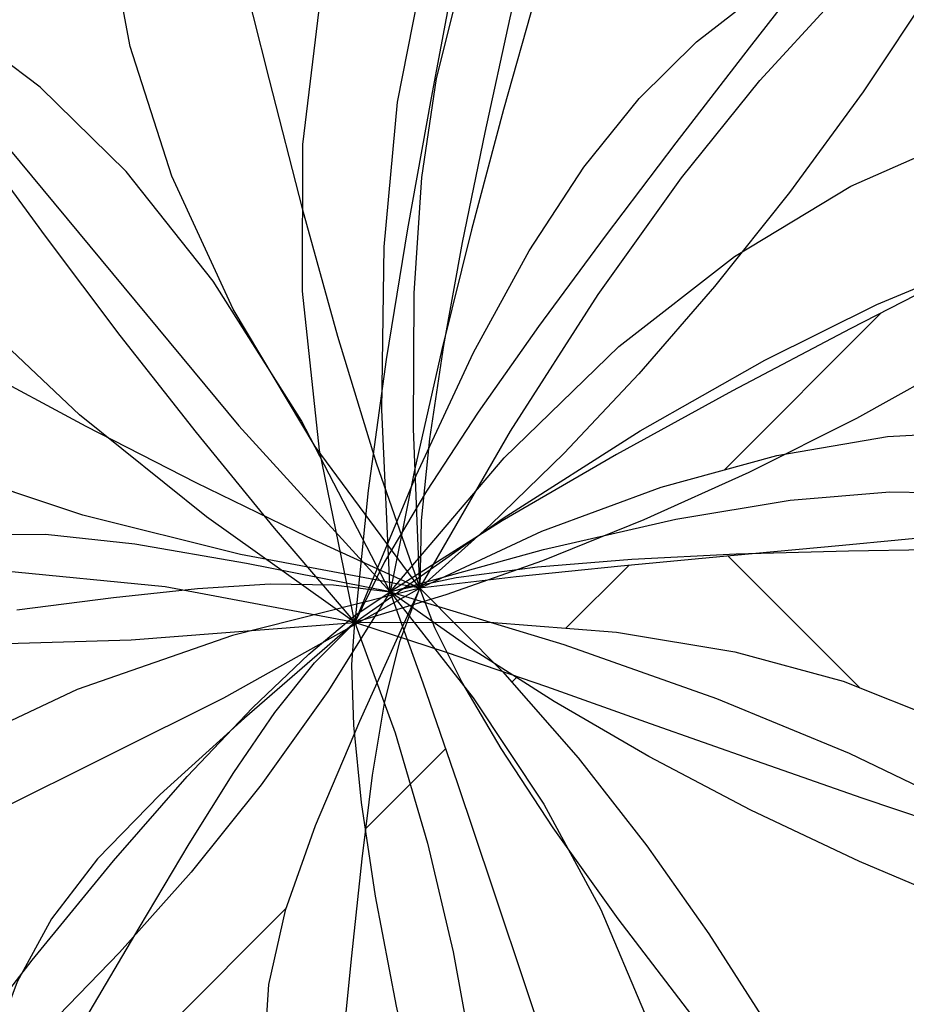
# Model space of a CAD drawing. Units: inches. Extents: x 3590 to 5167, y 65 to 1917.
# Tile 51 of 100: x 4947.17 to 4960.64, y 1515.58 to 1530.53. Entities that reach past the tile are written whole.
import ezdxf

# ---------------------------------------------------------------- set-up
doc = ezdxf.new("R2010")
doc.units = ezdxf.units.IN
doc.layers.add('A-FLOR-PATT', color=8, linetype='Continuous', lineweight=13)
doc.layers.add('L-PLNT', color=94, linetype='Continuous', lineweight=18)
doc.layers.add('DIENHOA', color=3, linetype='Continuous')

# ---------------------------------------------------------------- blocks, each defined once
blk = doc.blocks.new('Cay03_mb')
at = {"layer": 'DIENHOA'}
for p, q in [((9.94, 295.25), (25.49, 374.33)), ((96.72, 365.58), (75.6, 290.61)), ((-211.19, 304.6), (-263.5, 343.48)), ((-158.04, 252.34), (-211.19, 304.6)), ((1.62, 205.66), (9.94, 295.25)), ((75.6, 290.61), (55.75, 216.28)), ((-240.22, 277.83), (-88.39, 94.86)), ((290.63, 243.24), (363.38, 275.41)), ((-104.15, 184.39), (-158.04, 252.34)), ((218.51, 199.79), (290.63, 243.24)), ((55.75, 216.28), (37.33, 142.09)), ((0.21, 104.88), (1.62, 205.66)), ((146.96, 144.09), (218.51, 199.79)), ((363.69, 192.89), (290.19, 154.87)), ((-49.64, 98.45), (-104.15, 184.39)), ((290.19, 154.87), (217.38, 116.61)), ((37.33, 142.09), (20.49, 67.57)), ((75.94, 75.22), (146.96, 144.09)), ((217.38, 116.61), (145.48, 77.28)), ((5.39, -7.78), (0.21, 104.88)), ((5.39, -7.78), (-49.64, 98.45)), ((-88.39, 94.86), (5.39, -7.78)), ((5.39, -7.78), (75.94, 75.22)), ((145.48, 77.28), (74.74, 36.09)), ((20.49, 67.57), (5.39, -7.78)), ((182.2, 37.2), (252.97, 48.94)), ((252.97, 48.94), (314.63, 54.14)), ((314.63, 54.14), (369.18, 53.28)), ((100.34, 18.45), (182.2, 37.2)), ((74.74, 36.09), (5.39, -7.78)), ((-207.96, 27.76), (-254.73, 27.37)), ((-152.72, 21.72), (-207.96, 27.76)), ((-83.45, 9.72), (-152.72, 21.72)), ((5.39, -7.78), (100.34, 18.45)), ((361.61, 18.5), (289.03, 17.44)), ((154.97, 12.22), (96.66, 7.47)), ((219.62, 15.45), (154.97, 12.22)), ((289.03, 17.44), (219.62, 15.45)), ((5.39, -7.78), (-83.45, 9.72)), ((96.66, 7.47), (46.27, 0.9)), ((46.27, 0.9), (5.39, -7.78)), ((-165.8, -11.26), (-113.95, -5.74)), ((-113.95, -5.74), (-69, -2.91)), ((-69, -2.91), (-29.65, -3.38)), ((-29.65, -3.38), (5.39, -7.78)), ((-225.83, -18.85), (-165.8, -11.26)), ((5.39, -7.78), (-33.18, -69.47)), ((-16.51, -22.43), (5.39, -7.78)), ((5.39, -7.78), (56.83, -73.35)), ((25.88, -64.38), (5.39, -7.78)), ((5.39, -7.78), (112.81, -40.3)), ((53.47, -41.58), (5.39, -7.78)), ((-45.06, -46.34), (-16.51, -22.43)), ((106.98, -75.69), (53.47, -41.58)), ((112.81, -40.3), (207.46, -73.81)), ((-79.78, -79.55), (-45.06, -46.34)), ((47.05, -125.9), (25.88, -64.38)), ((-33.18, -69.47), (-74.57, -127.29)), ((56.83, -73.35), (100.42, -139.07)), ((165.52, -109.6), (106.98, -75.69)), ((207.46, -73.81), (289.55, -107.64)), ((-120.2, -122.13), (-79.78, -79.55)), ((228.67, -142.77), (165.52, -109.6)), ((289.55, -107.64), (359.29, -141.1)), ((-165.86, -174.12), (-120.2, -122.13)), ((-74.57, -127.29), (-117.85, -181.14)), ((68.74, -190.55), (47.05, -125.9)), ((100.42, -139.07), (135.85, -204.28)), ((296, -174.69), (228.67, -142.77)), ((-216.28, -235.58), (-165.86, -174.12)), ((367.1, -204.83), (296, -174.69)), ((-117.85, -181.14), (-162.07, -230.91)), ((90.79, -256.57), (68.74, -190.55)), ((135.85, -204.28), (162.8, -268.28)), ((-162.07, -230.91), (-206.29, -276.49)), ((-270.99, -306.55), (-216.28, -235.58)), ((113.06, -322.16), (90.79, -256.57))]:
    blk.add_line(p, q, dxfattribs=at)
for points in [[(23.69, -5.44), (-41, 82.2), (-91.83, 167.08), (-129.72, 249.45), (-155.55, 329.59), (-170.25, 407.76), (-174.71, 484.23), (-169.84, 559.26), (-156.54, 633.12)], [(-156.54, 633.12), (-132.46, 551.33), (-110.51, 470.02), (-89.84, 389.22), (-69.62, 308.98), (-48.99, 229.35), (-27.13, 150.38), (-3.18, 72.1), (23.69, -5.44)], [(-16.39, -26.73), (-38.34, 79.96), (-48.88, 178.33), (-48.7, 269), (-38.53, 352.58), (-19.08, 429.71), (8.95, 500.99), (44.86, 567.06), (87.92, 628.52)], [(87.92, 628.52), (75.46, 544.18), (61.27, 461.15), (46.13, 379.14), (30.83, 297.82), (16.14, 216.89), (2.85, 136.03), (-8.25, 54.92), (-16.39, -26.73)], [(23.69, -5.44), (19.84, 92.99), (20.28, 176.97), (25.02, 248.55), (34.03, 309.77), (47.33, 362.68), (64.91, 409.31), (86.75, 451.72), (112.87, 491.95)], [(112.87, 491.95), (95.99, 419.69), (79.46, 347.37), (63.92, 276.46), (50.01, 208.43), (38.38, 144.75), (29.69, 86.9), (24.57, 36.35), (23.69, -5.44)], [(-395.6, 473.65), (-347.51, 405.62), (-300.58, 339.5), (-254.33, 275.13), (-208.27, 212.32), (-161.92, 150.91), (-114.81, 90.72), (-66.46, 31.56), (-16.39, -26.73)], [(-16.39, -26.73), (-108.35, 38.55), (-186.88, 101.73), (-252.35, 163.45), (-305.09, 224.39), (-345.44, 285.22), (-373.75, 346.59), (-390.35, 409.18), (-395.6, 473.65)], [(384.28, 437.45), (342.25, 367.83), (298.14, 301.71), (252.56, 239.37), (206.11, 181.11), (159.39, 127.21), (113.01, 77.96), (67.57, 33.64), (23.69, -5.44)], [(23.69, -5.44), (79.88, 91.71), (134.12, 176.21), (185.81, 248.4), (234.31, 308.65), (279.02, 357.33), (319.33, 394.78), (354.62, 421.37), (384.28, 437.45)], [(273.24, 387.35), (227.6, 328.83), (182.25, 270.12), (138.39, 212.28), (97.23, 156.36), (59.96, 103.43), (27.8, 54.57), (1.94, 10.82), (-16.39, -26.73)], [(-16.39, -26.73), (21.41, 64.22), (57.05, 140.27), (91.37, 203.26), (125.24, 255.05), (159.51, 297.5), (195.03, 332.46), (232.65, 361.79), (273.24, 387.35)], [(-530.47, 289.69), (-458.27, 248.1), (-387.93, 207.77), (-318.94, 168.75), (-250.78, 131.06), (-182.94, 94.76), (-114.93, 59.88), (-46.22, 26.47), (23.69, -5.44)], [(23.69, -5.44), (-87.17, 15.25), (-184.97, 39.64), (-270.29, 68.2), (-343.73, 101.4), (-405.88, 139.68), (-457.33, 183.51), (-498.66, 233.36), (-530.47, 289.69)], [(496.74, 224.01), (429.38, 178.44), (361.6, 136.93), (294.07, 99.46), (227.46, 66.07), (162.44, 36.74), (99.68, 11.49), (39.84, -9.67), (-16.39, -26.73)], [(-16.39, -26.73), (75.38, 37.88), (160.06, 91.82), (237.27, 135.67), (306.57, 170.01), (367.58, 195.44), (419.88, 212.52), (463.07, 221.85), (496.74, 224.01)], [(23.69, -5.44), (99.27, 29.67), (173.22, 57.09), (244.79, 76.69), (313.26, 88.31), (377.88, 91.81), (437.93, 87.02), (492.67, 73.8), (541.37, 52)], [(541.37, 52), (484.11, 42.89), (421.18, 34.83), (354.36, 27.58), (285.41, 20.89), (216.1, 14.49), (148.2, 8.14), (83.47, 1.58), (23.69, -5.44)], [(-16.39, -26.73), (-133.98, -4.68), (-235.26, 5.29), (-321.98, 4.67), (-395.89, -5.03), (-458.73, -22.31), (-512.26, -45.67), (-558.22, -73.63), (-598.36, -104.66)], [(-471.89, -320.34), (-310.46, -179.32), (-97.66, -73.3), (23.69, -5.44)], [(23.69, -5.44), (-92.3, -34.76), (-188.42, -68.2), (-266.88, -105.14), (-329.9, -144.95), (-379.7, -187), (-418.48, -230.67), (-448.47, -275.32), (-471.89, -320.34)], [(23.69, -5.44), (-13.63, -87.94), (-41.14, -152.63), (-59.64, -205.04), (-69.94, -250.66), (-72.84, -295), (-69.17, -343.58), (-59.73, -401.89), (-45.32, -475.45)], [(-45.32, -475.45), (-34.09, -383.24), (-25.4, -302.82), (-18.34, -233.08), (-12.02, -172.9), (-5.55, -121.16), (1.96, -76.75), (11.41, -38.55), (23.69, -5.44)], [(316.49, -418.14), (251.44, -342.76), (194.84, -273.28), (146.52, -210.16), (106.33, -153.83), (74.11, -104.75), (49.71, -63.36), (32.95, -30.11), (23.69, -5.44)], [(23.69, -5.44), (74.94, -57.08), (121.78, -110.58), (164.32, -165.02), (202.67, -219.43), (236.95, -272.89), (267.27, -324.46), (293.75, -373.19), (316.49, -418.14)], [(-598.36, -104.66), (-392.67, -44.38), (-155.01, -37.42), (-16.39, -26.73)], [(-276.22, -424.43), (-227.35, -345.43), (-185.71, -276.08), (-150.05, -215.74), (-119.06, -163.76), (-91.49, -119.51), (-66.04, -82.35), (-41.43, -51.64), (-16.39, -26.73)], [(-16.39, -26.73), (-84.88, -85.96), (-136.99, -133.15), (-175.77, -172.96), (-204.26, -210.05), (-225.5, -249.08), (-242.55, -294.71), (-258.44, -351.61), (-276.22, -424.43)], [(76.25, -524.2), (48.83, -428.48), (26.6, -341.67), (9.22, -264.1), (-3.63, -196.11), (-12.28, -138.04), (-17.07, -90.23), (-18.33, -53.01), (-16.39, -26.73)], [(-16.39, -26.73), (66.95, -26.58), (145.58, -32.71), (218.77, -44.94), (285.79, -63.12), (345.92, -87.06), (398.42, -116.6), (442.57, -151.57), (477.63, -191.79)], [(477.63, -191.79), (421.82, -176.03), (361.32, -156.94), (297.62, -135.49), (232.22, -112.64), (166.63, -89.37), (102.33, -66.65), (40.82, -45.45), (-16.39, -26.73)], [(-16.39, -26.73), (8.47, -95.11), (28.54, -163.33), (44.32, -230.59), (56.3, -296.08), (64.99, -358.99), (70.88, -418.52), (74.46, -473.86), (76.25, -524.2)]]:
    blk.add_lwpolyline(points, dxfattribs=at)

msp = doc.modelspace()

# ---------------------------------------------------------------- hatches: boundary and pattern name
at = {"layer": 'A-FLOR-PATT', "transparency": 33554687}
h = msp.add_hatch(dxfattribs=at)
h.set_pattern_fill('AR-HBONE', color=256, scale=0.2)
h.set_pattern_definition([(45, (-588.972, 0), (0, 28.73682), [60.96, -20.32]), (135, (-574.604, 14.368), (3e-15, 28.73682), [60.96, -20.32])])
h.paths.add_polyline_path([(5071.274, 1796.999), (4933.274, 1796.999), (4933.274, 1753.999), (4962.774, 1753.999, -0.414214), (4928.774, 1719.999), (4933.274, 1718.999), (4933.274, 1334.999), (5071.274, 1334.999)])
h.paths.add_polyline_path([(4951.78, 1521.077), (4951.715, 1521.04), (4951.563, 1520.895)], flags=16)
h.paths.add_polyline_path([(4952.267, 1521.376), (4952.198, 1521.371), (4952.198, 1521.356)], flags=0)
h.paths.add_polyline_path([(4967.051, 1529.728), (4965.231, 1528.694), (4963.411, 1527.714), (4961.756, 1526.851), (4963.589, 1527.449), (4964.036, 1527.478), (4962.975, 1527.249), (4961.76, 1526.852), (4959.792, 1525.834), (4958.005, 1524.895), (4956.24, 1523.93), (4954.504, 1522.919), (4954.129, 1522.682), (4953.361, 1521.997), (4953.366, 1521.998), (4953.605, 1522.064), (4955.106, 1522.761), (4956.921, 1523.434), (4958.678, 1523.915), (4960.358, 1524.2), (4961.945, 1524.286), (4964.171, 1524.108), (4965.958, 1523.309), (4963.863, 1522.976), (4965.187, 1522.499), (4963.366, 1522.497), (4961.545, 1522.487), (4959.764, 1522.461), (4958.304, 1522.419), (4957.974, 1522.388), (4956.307, 1522.232), (4954.718, 1522.071), (4953.251, 1521.899), (4953.525, 1521.623), (4954.331, 1521.379), (4956.243, 1521.23), (4958.039, 1520.93), (4959.684, 1520.483), (4961.16, 1519.896), (4963.107, 1518.8), (4964.393, 1517.325), (4962.973, 1517.726), (4964.558, 1516.661), (4965.407, 1515.708), (4963.507, 1516.322), (4961.68, 1517.005), (4959.935, 1517.745), (4958.282, 1518.528), (4956.732, 1519.343), (4955.295, 1520.175), (4954.672, 1520.572), (4954.513, 1520.627), (4955.658, 1519.318), (4956.703, 1517.982), (4957.644, 1516.647), (4958.485, 1515.334), (4959.55, 1513.524), (4960.438, 1511.769), (4958.841, 1513.62), (4957.452, 1515.325), (4955.819, 1517.459), (4956.665, 1515.448), (4957.111, 1513.923), (4957.447, 1511.714), (4957.076, 1509.793), (4956.538, 1511.11), (4955.992, 1512.569), (4955.444, 1514.125), (4954.898, 1515.735), (4954.357, 1517.356), (4953.824, 1518.943), (4953.305, 1520.452), (4953.065, 1521.116), (4952.971, 1521.146), (4952.949, 1521.086), (4952.73, 1520.199), (4953.37, 1518.024), (4953.757, 1516.373), (4954.051, 1514.765), (4954.264, 1513.221), (4954.471, 1511.131), (4954.497, 1510.402), (4954.409, 1511.76), (4954.264, 1513.221), (4954.051, 1514.765), (4953.757, 1516.373), (4953.37, 1518.024), (4952.877, 1519.698), (4952.716, 1520.141), (4952.533, 1519.059), (4952.374, 1517.789), (4952.219, 1516.312), (4952.046, 1514.6), (4951.833, 1512.626), (4951.557, 1510.363), (4951.203, 1512.168), (4950.852, 1514.339), (4950.985, 1516.376), (4951.66, 1518.286), (4952.593, 1520.481), (4952.357, 1521.13), (4951.855, 1520.328), (4950.839, 1518.908), (4949.777, 1517.587), (4948.916, 1516.617), (4948.111, 1515.256), (4947.089, 1513.554), (4945.889, 1511.615), (4946.326, 1513.402), (4946.562, 1514.249), (4945.528, 1513.327), (4944.581, 1512.531), (4946.018, 1514.508), (4947.204, 1516.048), (4947.893, 1517.313), (4949.307, 1518.764), (4950.414, 1519.767), (4950.451, 1519.806), (4952.267, 1521.376), (4951.645, 1521.493), (4950.404, 1521.18), (4948.044, 1520.359), (4946.119, 1519.452), (4944.572, 1518.475), (4943.35, 1517.443), (4941.997, 1515.92), (4941.661, 1515.275), (4942.813, 1516.99), (4944.572, 1518.475), (4946.119, 1519.452), (4948.044, 1520.359), (4950.404, 1521.18), (4951.645, 1521.493), (4949.647, 1521.868), (4948.6, 1521.756), (4947.126, 1521.57), (4945.42, 1521.348), (4943.45, 1521.105), (4941.183, 1520.856), (4942.86, 1521.613), (4943.873, 1522.03), (4942.952, 1521.909), (4941.41, 1521.485), (4939.543, 1520.67), (4938.968, 1520.226), (4940.733, 1521.299), (4942.952, 1521.909), (4943.702, 1522.008), (4945.894, 1522.7), (4947.565, 1522.714), (4948.921, 1522.566), (4951.131, 1522.183), (4950.971, 1522.297), (4948.129, 1523.006), (4946.035, 1523.707), (4944.232, 1524.521), (4942.707, 1525.461), (4941.444, 1526.537), (4940.43, 1527.761), (4939.649, 1529.143), (4941.421, 1528.122), (4943.147, 1527.132), (4944.841, 1526.175), (4946.514, 1525.25), (4948.179, 1524.359), (4948.365, 1524.263), (4946.475, 1526.045), (4945.181, 1527.54), (4944.19, 1529.033), (4943.496, 1530.54), (4943.278, 1531.36), (4942.498, 1531.919), (4943.114, 1531.762), (4942.959, 1533.659), (4944.14, 1531.989), (4944.612, 1531.323), (4946.202, 1530.463), (4947.486, 1529.509), (4948.79, 1528.226), (4950.368, 1526.237), (4949.485, 1528.155), (4948.851, 1530.123), (4948.491, 1532.041), (4948.381, 1533.918), (4948.501, 1535.76), (4948.827, 1537.573), (4949.418, 1535.565), (4949.957, 1533.569), (4950.464, 1531.586), (4950.961, 1529.617), (4951.391, 1527.954), (4951.724, 1530.687), (4952.201, 1532.58), (4952.889, 1534.33), (4953.77, 1535.951), (4954.827, 1537.46), (4954.521, 1535.39), (4954.273, 1533.937), (4955.58, 1535.663), (4956.748, 1536.739), (4956.159, 1534.78), (4955.589, 1532.873), (4955.043, 1531.006), (4954.525, 1529.166), (4954.038, 1527.341), (4953.638, 1525.733), (4953.611, 1525.586), (4953.398, 1524.166), (4953.382, 1524.009), (4954.07, 1525.476), (4954.912, 1527.022), (4956.136, 1528.894), (4957.847, 1530.577), (4959.376, 1531.54), (4958.256, 1530.104), (4957.143, 1528.663), (4956.066, 1527.243), (4955.056, 1525.871), (4954.141, 1524.571), (4953.352, 1523.372), (4953.311, 1523.303), (4953.273, 1522.925), (4953.261, 1522.382), (4954.103, 1523.373), (4954.63, 1524.284), (4955.961, 1526.358), (4957.23, 1528.13), (4958.421, 1529.609), (4960.037, 1531.368), (4961.374, 1532.375), (4962.101, 1532.77), (4961.07, 1531.061), (4959.987, 1529.438), (4958.869, 1527.908), (4958.15, 1527.007), (4959.803, 1528.003), (4961.589, 1528.793), (4963.391, 1529.328), (4965.211, 1529.632)], flags=16)
h.paths.add_polyline_path([(4962.944, 1523.182), (4961.107, 1523.422), (4960.392, 1523.362), (4962.35, 1523.331)], flags=0)
h.paths.add_polyline_path([(5049.541, 1584.551), (5049.476, 1584.515), (5049.325, 1584.37)], flags=16)
h.paths.add_polyline_path([(5050.028, 1584.851), (5049.959, 1584.845), (5049.959, 1584.83)], flags=0)
h.paths.add_polyline_path([(5042.333, 1581.949), (5043.88, 1582.926), (5045.806, 1583.833), (5048.165, 1584.654), (5049.406, 1584.967), (5047.408, 1585.342), (5046.361, 1585.231), (5044.888, 1585.044), (5043.181, 1584.822), (5041.211, 1584.579), (5038.944, 1584.33), (5040.622, 1585.087), (5041.634, 1585.504), (5040.713, 1585.383), (5039.171, 1584.959), (5037.304, 1584.144), (5036.729, 1583.7), (5038.494, 1584.773), (5040.713, 1585.383), (5041.463, 1585.482), (5043.655, 1586.174), (5045.326, 1586.188), (5046.682, 1586.04), (5048.893, 1585.657), (5048.732, 1585.771), (5045.891, 1586.48), (5043.796, 1587.181), (5041.994, 1587.996), (5040.468, 1588.935), (5039.205, 1590.011), (5038.191, 1591.235), (5037.41, 1592.617), (5039.182, 1591.596), (5040.909, 1590.607), (5042.602, 1589.649), (5044.275, 1588.724), (5045.94, 1587.833), (5046.126, 1587.738), (5044.237, 1589.519), (5042.942, 1591.015), (5041.952, 1592.508), (5041.257, 1594.014), (5041.039, 1594.834), (5040.26, 1595.393), (5040.875, 1595.237), (5040.721, 1597.133), (5041.901, 1595.463), (5042.373, 1594.798), (5043.963, 1593.938), (5045.247, 1592.983), (5046.552, 1591.701), (5048.129, 1589.712), (5047.247, 1591.63), (5046.613, 1593.597), (5046.252, 1595.515), (5046.142, 1597.392), (5046.262, 1599.234), (5046.588, 1601.047), (5047.179, 1599.039), (5047.718, 1597.043), (5048.225, 1595.06), (5048.722, 1593.091), (5049.152, 1591.429), (5049.485, 1594.161), (5049.962, 1596.054), (5050.65, 1597.804), (5051.532, 1599.425), (5052.589, 1600.934), (5052.283, 1598.864), (5052.034, 1597.411), (5053.341, 1599.137), (5054.509, 1600.213), (5053.92, 1598.254), (5053.35, 1596.348), (5052.805, 1594.48), (5052.286, 1592.64), (5051.799, 1590.815), (5051.4, 1589.207), (5051.373, 1589.06), (5051.159, 1587.64), (5051.143, 1587.483), (5051.831, 1588.95), (5052.673, 1590.496), (5053.898, 1592.368), (5055.608, 1594.051), (5057.137, 1595.014), (5056.017, 1593.578), (5054.904, 1592.137), (5053.828, 1590.717), (5052.817, 1589.345), (5051.902, 1588.046), (5051.113, 1586.846), (5051.072, 1586.777), (5051.034, 1586.399), (5051.022, 1585.856), (5051.864, 1586.847), (5052.391, 1587.758), (5053.723, 1589.832), (5054.991, 1591.604), (5056.182, 1593.083), (5057.798, 1594.842), (5059.135, 1595.849), (5059.863, 1596.244), (5058.831, 1594.535), (5057.749, 1592.912), (5056.63, 1591.382), (5055.912, 1590.482), (5057.564, 1591.477), (5059.35, 1592.267), (5061.152, 1592.802), (5062.972, 1593.106), (5064.812, 1593.203), (5062.992, 1592.169), (5061.172, 1591.188), (5059.518, 1590.325), (5061.35, 1590.924), (5061.797, 1590.952), (5060.737, 1590.723), (5059.521, 1590.326), (5057.553, 1589.308), (5055.766, 1588.369), (5054.002, 1587.404), (5052.265, 1586.393), (5051.891, 1586.156), (5051.122, 1585.471), (5051.127, 1585.472), (5051.366, 1585.538), (5052.867, 1586.235), (5054.682, 1586.908), (5056.439, 1587.389), (5058.12, 1587.675), (5059.706, 1587.76), (5061.933, 1587.583), (5063.719, 1586.783), (5061.624, 1586.45), (5062.949, 1585.973), (5061.127, 1585.971), (5059.307, 1585.961), (5057.525, 1585.935), (5056.065, 1585.893), (5055.735, 1585.862), (5054.068, 1585.707), (5052.479, 1585.546), (5051.012, 1585.373), (5051.286, 1585.097), (5052.092, 1584.853), (5054.004, 1584.704), (5055.8, 1584.404), (5057.446, 1583.958), (5058.921, 1583.37), (5060.868, 1582.274), (5062.154, 1580.799), (5060.734, 1581.2), (5062.32, 1580.135), (5063.168, 1579.182), (5061.269, 1579.796), (5059.441, 1580.479), (5057.696, 1581.219), (5056.043, 1582.003), (5054.493, 1582.817), (5053.057, 1583.649), (5052.433, 1584.047), (5052.274, 1584.101), (5053.42, 1582.793), (5054.464, 1581.457), (5055.405, 1580.121), (5056.247, 1578.809), (5057.311, 1576.998), (5058.199, 1575.244), (5056.602, 1577.094), (5055.213, 1578.799), (5053.58, 1580.933), (5054.427, 1578.922), (5054.872, 1577.397), (5055.208, 1575.189), (5054.838, 1573.267), (5054.299, 1574.584), (5053.754, 1576.043), (5053.206, 1577.599), (5052.659, 1579.209), (5052.118, 1580.83), (5051.585, 1582.417), (5051.066, 1583.927), (5050.826, 1584.59), (5050.733, 1584.62), (5050.711, 1584.561), (5050.491, 1583.673), (5051.131, 1581.498), (5051.518, 1579.847), (5051.813, 1578.24), (5052.026, 1576.695), (5052.233, 1574.605), (5052.258, 1573.876), (5052.17, 1575.234), (5052.026, 1576.695), (5051.813, 1578.24), (5051.518, 1579.847), (5051.131, 1581.498), (5050.638, 1583.172), (5050.477, 1583.615), (5050.294, 1582.533), (5050.136, 1581.263), (5049.981, 1579.786), (5049.807, 1578.074), (5049.594, 1576.1), (5049.318, 1573.837), (5048.965, 1575.642), (5048.613, 1577.813), (5048.747, 1579.85), (5049.421, 1581.76), (5050.354, 1583.955), (5050.118, 1584.604), (5049.616, 1583.802), (5048.6, 1582.382), (5047.538, 1581.061), (5046.677, 1580.091), (5045.872, 1578.73), (5044.85, 1577.028), (5043.651, 1575.089), (5044.087, 1576.877), (5044.324, 1577.723), (5043.289, 1576.801), (5042.342, 1576.005), (5043.779, 1577.982), (5044.966, 1579.522), (5045.655, 1580.787), (5047.068, 1582.239), (5048.175, 1583.241), (5048.213, 1583.28), (5050.028, 1584.851), (5049.406, 1584.967), (5048.165, 1584.654), (5045.806, 1583.833), (5043.88, 1582.926), (5042.333, 1581.949), (5041.111, 1580.917), (5039.758, 1579.394), (5039.423, 1578.749), (5040.575, 1580.464)], flags=16)
h.paths.add_polyline_path([(4954.799, 1533.12), (4954.262, 1532.079), (4953.831, 1530.935), (4953.505, 1529.636), (4953.283, 1528.133), (4953.167, 1526.376), (4953.156, 1524.315), (4953.277, 1521.236), (4952.802, 1521.842), (4951.557, 1521.998), (4950.976, 1521.961), (4952.661, 1521.941), (4952.802, 1521.842), (4953.152, 1523.593), (4953.167, 1526.376), (4953.283, 1528.133), (4953.609, 1530.346), (4954.456, 1532.592)], flags=0)
h.paths.add_polyline_path([(5050.563, 1585.316), (5049.318, 1585.472), (5048.737, 1585.435), (5050.422, 1585.415), (5050.563, 1585.316), (5050.914, 1587.067), (5050.928, 1589.851), (5051.045, 1591.607), (5051.371, 1593.82), (5052.217, 1596.066), (5052.56, 1596.594), (5052.024, 1595.554), (5051.592, 1594.409), (5051.266, 1593.11), (5051.045, 1591.607), (5050.928, 1589.851), (5050.918, 1587.789), (5051.038, 1584.71)], flags=0)
h.paths.add_polyline_path([(5058.153, 1586.836), (5060.111, 1586.805), (5060.705, 1586.656), (5058.868, 1586.896)], flags=0)
h.paths.add_polyline_path([(5049.541, 1430.936), (5049.476, 1430.9), (5049.325, 1430.755)], flags=16)
h.paths.add_polyline_path([(5050.028, 1431.236), (5049.959, 1431.231), (5049.959, 1431.215)], flags=0)
h.paths.add_polyline_path([(5046.588, 1447.432), (5047.179, 1445.425), (5047.718, 1443.429), (5048.225, 1441.446), (5048.722, 1439.476), (5049.152, 1437.814), (5049.485, 1440.546), (5049.962, 1442.439), (5050.65, 1444.189), (5051.532, 1445.811), (5052.589, 1447.319), (5052.283, 1445.249), (5052.034, 1443.796), (5053.341, 1445.522), (5054.509, 1446.598), (5053.92, 1444.64), (5053.35, 1442.733), (5052.805, 1440.865), (5052.286, 1439.025), (5051.799, 1437.201), (5051.4, 1435.592), (5051.373, 1435.445), (5051.159, 1434.025), (5051.143, 1433.868), (5051.831, 1435.335), (5052.673, 1436.881), (5053.898, 1438.753), (5055.608, 1440.436), (5057.137, 1441.4), (5056.017, 1439.963), (5054.904, 1438.522), (5053.828, 1437.102), (5052.817, 1435.73), (5051.902, 1434.431), (5051.113, 1433.231), (5051.072, 1433.162), (5051.034, 1432.784), (5051.022, 1432.242), (5051.864, 1433.232), (5052.391, 1434.143), (5053.723, 1436.217), (5054.991, 1437.989), (5056.182, 1439.468), (5057.798, 1441.227), (5059.135, 1442.235), (5059.863, 1442.629), (5058.831, 1440.921), (5057.749, 1439.298), (5056.63, 1437.767), (5055.912, 1436.867), (5057.564, 1437.863), (5059.35, 1438.652), (5061.152, 1439.187), (5062.972, 1439.491), (5064.812, 1439.588), (5062.992, 1438.554), (5061.172, 1437.573), (5059.518, 1436.71), (5061.35, 1437.309), (5061.797, 1437.337), (5060.737, 1437.108), (5059.521, 1436.711), (5057.553, 1435.693), (5055.766, 1434.754), (5054.002, 1433.789), (5052.265, 1432.778), (5051.891, 1432.541), (5051.122, 1431.856), (5051.127, 1431.857), (5051.366, 1431.923), (5052.867, 1432.62), (5054.682, 1433.293), (5056.439, 1433.775), (5058.12, 1434.06), (5059.706, 1434.145), (5061.933, 1433.968), (5063.719, 1433.168), (5061.624, 1432.835), (5062.949, 1432.358), (5061.127, 1432.357), (5059.307, 1432.346), (5057.525, 1432.32), (5056.065, 1432.278), (5055.735, 1432.248), (5054.068, 1432.092), (5052.479, 1431.931), (5051.012, 1431.759), (5051.286, 1431.482), (5052.092, 1431.238), (5054.004, 1431.089), (5055.8, 1430.789), (5057.446, 1430.343), (5058.921, 1429.755), (5060.868, 1428.66), (5062.154, 1427.185), (5060.734, 1427.585), (5062.32, 1426.52), (5063.168, 1425.567), (5061.269, 1426.181), (5059.441, 1426.865), (5057.696, 1427.604), (5056.043, 1428.388), (5054.493, 1429.202), (5053.057, 1430.034), (5052.433, 1430.432), (5052.274, 1430.487), (5053.42, 1429.178), (5054.464, 1427.842), (5055.405, 1426.506), (5056.247, 1425.194), (5057.311, 1423.383), (5058.199, 1421.629), (5056.602, 1423.479), (5055.213, 1425.184), (5053.58, 1427.318), (5054.427, 1425.307), (5054.872, 1423.782), (5055.208, 1421.574), (5054.838, 1419.652), (5054.299, 1420.97), (5053.754, 1422.428), (5053.206, 1423.984), (5052.659, 1425.595), (5052.118, 1427.215), (5051.585, 1428.802), (5051.066, 1430.312), (5050.826, 1430.975), (5050.733, 1431.005), (5050.711, 1430.946), (5050.491, 1430.058), (5051.131, 1427.883), (5051.518, 1426.232), (5051.813, 1424.625), (5052.026, 1423.081), (5052.233, 1420.991), (5052.258, 1420.261), (5052.17, 1421.619), (5052.026, 1423.081), (5051.813, 1424.625), (5051.518, 1426.232), (5051.131, 1427.883), (5050.638, 1429.558), (5050.477, 1430.001), (5050.294, 1428.918), (5050.136, 1427.648), (5049.981, 1426.171), (5049.807, 1424.459), (5049.594, 1422.485), (5049.318, 1420.222), (5048.965, 1422.028), (5048.613, 1424.199), (5048.747, 1426.235), (5049.421, 1428.146), (5050.354, 1430.34), (5050.118, 1430.989), (5049.616, 1430.187), (5048.6, 1428.768), (5047.538, 1427.446), (5046.677, 1426.477), (5045.872, 1425.116), (5044.85, 1423.413), (5043.651, 1421.474), (5044.087, 1423.262), (5044.324, 1424.109), (5043.289, 1423.186), (5042.342, 1422.391), (5043.779, 1424.368), (5044.966, 1425.907), (5045.655, 1427.173), (5047.068, 1428.624), (5048.175, 1429.627), (5048.213, 1429.666), (5050.028, 1431.236), (5049.406, 1431.353), (5048.165, 1431.039), (5045.806, 1430.218), (5043.88, 1429.311), (5042.333, 1428.334), (5041.111, 1427.302), (5039.758, 1425.779), (5039.423, 1425.134), (5040.575, 1426.849), (5042.333, 1428.334), (5043.88, 1429.311), (5045.806, 1430.218), (5048.165, 1431.039), (5049.406, 1431.353), (5047.408, 1431.727), (5046.361, 1431.616), (5044.888, 1431.429), (5043.181, 1431.207), (5041.211, 1430.964), (5038.944, 1430.715), (5040.622, 1431.472), (5041.634, 1431.89), (5040.713, 1431.769), (5039.171, 1431.345), (5037.304, 1430.53), (5036.729, 1430.085), (5038.494, 1431.158), (5040.713, 1431.769), (5041.463, 1431.867), (5043.655, 1432.559), (5045.326, 1432.573), (5046.682, 1432.425), (5048.893, 1432.042), (5048.732, 1432.156), (5045.891, 1432.865), (5043.796, 1433.566), (5041.994, 1434.381), (5040.468, 1435.321), (5039.205, 1436.396), (5038.191, 1437.62), (5037.41, 1439.002), (5039.182, 1437.982), (5040.909, 1436.992), (5042.602, 1436.034), (5044.275, 1435.109), (5045.94, 1434.218), (5046.126, 1434.123), (5044.237, 1435.904), (5042.942, 1437.4), (5041.952, 1438.893), (5041.257, 1440.399), (5041.039, 1441.219), (5040.26, 1441.778), (5040.875, 1441.622), (5040.721, 1443.518), (5041.901, 1441.848), (5042.373, 1441.183), (5043.963, 1440.323), (5045.247, 1439.369), (5046.552, 1438.086), (5048.129, 1436.097), (5047.247, 1438.015), (5046.613, 1439.982), (5046.252, 1441.901), (5046.142, 1443.778), (5046.262, 1445.619)], flags=16)
h.paths.add_polyline_path([(5052.382, 1444.255), (5051.623, 1442.78), (5052.024, 1441.939), (5052.56, 1442.98)], flags=0)
h.paths.add_polyline_path([(5050.563, 1431.701), (5049.318, 1431.857), (5048.737, 1431.821), (5050.422, 1431.8)], flags=0)
h.paths.add_polyline_path([(5058.153, 1433.221), (5060.111, 1433.19), (5060.705, 1433.041), (5058.868, 1433.281)], flags=0)
h.paths.add_polyline_path([(5049.541, 1352.285), (5049.476, 1352.249), (5049.325, 1352.104)], flags=16)
h.paths.add_polyline_path([(5050.028, 1352.585), (5049.959, 1352.58), (5049.959, 1352.564)], flags=0)
h.paths.add_polyline_path([(5046.588, 1368.781), (5047.179, 1366.774), (5047.718, 1364.778), (5048.225, 1362.795), (5048.722, 1360.825), (5049.152, 1359.163), (5049.485, 1361.896), (5049.962, 1363.789), (5050.65, 1365.538), (5051.532, 1367.16), (5052.589, 1368.669), (5052.283, 1366.598), (5052.034, 1365.145), (5053.341, 1366.871), (5054.509, 1367.947), (5053.92, 1365.989), (5053.35, 1364.082), (5052.805, 1362.214), (5052.286, 1360.374), (5051.799, 1358.55), (5051.4, 1356.942), (5051.373, 1356.794), (5051.159, 1355.374), (5051.143, 1355.218), (5051.831, 1356.684), (5052.673, 1358.23), (5053.898, 1360.102), (5055.608, 1361.786), (5057.137, 1362.749), (5056.017, 1361.313), (5054.904, 1359.872), (5053.828, 1358.452), (5052.817, 1357.079), (5051.902, 1355.78), (5051.113, 1354.581), (5051.072, 1354.512), (5051.034, 1354.133), (5051.022, 1353.591), (5051.864, 1354.581), (5052.391, 1355.492), (5053.723, 1357.566), (5054.991, 1359.338), (5056.182, 1360.817), (5057.798, 1362.577), (5059.135, 1363.584), (5059.863, 1363.979), (5058.831, 1362.27), (5057.749, 1360.647), (5056.63, 1359.117), (5055.912, 1358.216), (5057.564, 1359.212), (5059.35, 1360.001), (5061.152, 1360.536), (5062.972, 1360.841), (5064.812, 1360.937), (5062.992, 1359.903), (5061.172, 1358.923), (5059.518, 1358.059), (5061.35, 1358.658), (5061.797, 1358.687), (5060.737, 1358.458), (5059.521, 1358.061), (5057.553, 1357.043), (5055.766, 1356.103), (5054.002, 1355.138), (5052.265, 1354.127), (5051.891, 1353.89), (5051.122, 1353.206), (5051.127, 1353.206), (5051.366, 1353.272), (5052.867, 1353.969), (5054.682, 1354.643), (5056.439, 1355.124), (5058.12, 1355.409), (5059.706, 1355.495), (5061.933, 1355.317), (5063.719, 1354.518), (5061.624, 1354.184), (5062.949, 1353.708), (5061.127, 1353.706), (5059.307, 1353.695), (5057.525, 1353.669), (5056.065, 1353.627), (5055.735, 1353.597), (5054.068, 1353.441), (5052.479, 1353.28), (5051.012, 1353.108), (5051.286, 1352.831), (5052.092, 1352.587), (5054.004, 1352.439), (5055.8, 1352.138), (5057.446, 1351.692), (5058.921, 1351.104), (5060.868, 1350.009), (5062.154, 1348.534), (5060.734, 1348.935), (5062.32, 1347.869), (5063.168, 1346.916), (5061.269, 1347.53), (5059.441, 1348.214), (5057.696, 1348.954), (5056.043, 1349.737), (5054.493, 1350.551), (5053.057, 1351.383), (5052.433, 1351.781), (5052.274, 1351.836), (5053.42, 1350.527), (5054.464, 1349.191), (5055.405, 1347.855), (5056.247, 1346.543), (5057.311, 1344.733), (5058.199, 1342.978), (5056.602, 1344.828), (5055.213, 1346.534), (5053.58, 1348.667), (5054.427, 1346.656), (5054.872, 1345.132), (5055.208, 1342.923), (5054.838, 1341.002), (5054.299, 1342.319), (5053.754, 1343.778), (5053.206, 1345.334), (5052.659, 1346.944), (5052.118, 1348.564), (5051.585, 1350.151), (5051.066, 1351.661), (5050.826, 1352.324), (5050.733, 1352.355), (5050.711, 1352.295), (5050.491, 1351.408), (5051.131, 1349.232), (5051.518, 1347.581), (5051.813, 1345.974), (5052.026, 1344.43), (5052.233, 1342.34), (5052.258, 1341.61), (5052.17, 1342.969), (5052.026, 1344.43), (5051.813, 1345.974), (5051.518, 1347.581), (5051.131, 1349.232), (5050.638, 1350.907), (5050.477, 1351.35), (5050.294, 1350.267), (5050.136, 1348.997), (5049.981, 1347.52), (5049.807, 1345.809), (5049.594, 1343.835), (5049.318, 1341.571), (5048.965, 1343.377), (5048.613, 1345.548), (5048.747, 1347.585), (5049.421, 1349.495), (5050.354, 1351.689), (5050.118, 1352.339), (5049.616, 1351.536), (5048.6, 1350.117), (5047.538, 1348.795), (5046.677, 1347.826), (5045.872, 1346.465), (5044.85, 1344.763), (5043.651, 1342.824), (5044.087, 1344.611), (5044.324, 1345.458), (5043.289, 1344.535), (5042.342, 1343.74), (5043.779, 1345.717), (5044.966, 1347.256), (5045.655, 1348.522), (5047.068, 1349.973), (5048.175, 1350.976), (5048.213, 1351.015), (5050.028, 1352.585), (5049.406, 1352.702), (5048.165, 1352.388), (5045.806, 1351.567), (5043.88, 1350.661), (5042.333, 1349.683), (5041.111, 1348.651), (5039.758, 1347.128), (5039.423, 1346.483), (5040.575, 1348.198), (5042.333, 1349.683), (5043.88, 1350.661), (5045.806, 1351.567), (5048.165, 1352.388), (5049.406, 1352.702), (5047.408, 1353.076), (5046.361, 1352.965), (5044.888, 1352.779), (5043.181, 1352.556), (5041.211, 1352.313), (5038.944, 1352.065), (5040.622, 1352.821), (5041.634, 1353.239), (5040.713, 1353.118), (5039.171, 1352.694), (5037.304, 1351.879), (5036.729, 1351.434), (5038.494, 1352.508), (5040.713, 1353.118), (5041.463, 1353.216), (5043.655, 1353.909), (5045.326, 1353.923), (5046.682, 1353.774), (5048.893, 1353.391), (5048.732, 1353.506), (5045.891, 1354.214), (5043.796, 1354.915), (5041.994, 1355.73), (5040.468, 1356.67), (5039.205, 1357.746), (5038.191, 1358.969), (5037.41, 1360.352), (5039.182, 1359.331), (5040.909, 1358.341), (5042.602, 1357.383), (5044.275, 1356.458), (5045.94, 1355.567), (5046.126, 1355.472), (5044.237, 1357.253), (5042.942, 1358.749), (5041.952, 1360.242), (5041.257, 1361.748), (5041.039, 1362.568), (5040.26, 1363.128), (5040.875, 1362.971), (5040.721, 1364.867), (5041.901, 1363.197), (5042.373, 1362.532), (5043.963, 1361.672), (5045.247, 1360.718), (5046.552, 1359.435), (5048.129, 1357.446), (5047.247, 1359.364), (5046.613, 1361.331), (5046.252, 1363.25), (5046.142, 1365.127), (5046.262, 1366.969)], flags=16)
h.paths.add_polyline_path([(5052.382, 1365.604), (5051.623, 1364.129), (5052.024, 1363.288), (5052.56, 1364.329)], flags=0)
h.paths.add_polyline_path([(4951.78, 1698.041), (4951.715, 1698.005), (4951.563, 1697.859)], flags=16)
h.paths.add_polyline_path([(4952.267, 1698.341), (4952.198, 1698.335), (4952.198, 1698.32)], flags=0)
h.paths.add_polyline_path([(4957.076, 1686.757), (4956.538, 1688.074), (4955.992, 1689.533), (4955.444, 1691.089), (4954.898, 1692.699), (4954.357, 1694.32), (4953.824, 1695.907), (4953.305, 1697.417), (4953.065, 1698.08), (4952.971, 1698.11), (4952.949, 1698.051), (4952.73, 1697.163), (4953.37, 1694.988), (4953.757, 1693.337), (4954.051, 1691.729), (4954.264, 1690.185), (4954.471, 1688.095), (4954.497, 1687.366), (4954.409, 1688.724), (4954.264, 1690.185), (4954.051, 1691.729), (4953.757, 1693.337), (4953.37, 1694.988), (4952.877, 1696.662), (4952.716, 1697.105), (4952.533, 1696.023), (4952.374, 1694.753), (4952.219, 1693.276), (4952.046, 1691.564), (4951.833, 1689.59), (4951.557, 1687.327), (4951.203, 1689.132), (4950.852, 1691.303), (4950.985, 1693.34), (4951.66, 1695.25), (4952.593, 1697.445), (4952.357, 1698.094), (4951.855, 1697.292), (4950.839, 1695.872), (4949.777, 1694.551), (4948.916, 1693.581), (4948.111, 1692.22), (4947.089, 1690.518), (4945.889, 1688.579), (4946.326, 1690.366), (4946.562, 1691.213), (4945.528, 1690.291), (4944.581, 1689.495), (4946.018, 1691.472), (4947.204, 1693.012), (4947.893, 1694.277), (4949.307, 1695.729), (4950.414, 1696.731), (4950.451, 1696.77), (4952.267, 1698.341), (4951.645, 1698.457), (4950.404, 1698.144), (4948.044, 1697.323), (4946.119, 1696.416), (4944.572, 1695.439), (4943.35, 1694.407), (4941.997, 1692.884), (4941.661, 1692.239), (4942.813, 1693.954), (4944.572, 1695.439), (4946.119, 1696.416), (4948.044, 1697.323), (4950.404, 1698.144), (4951.645, 1698.457), (4949.647, 1698.832), (4948.6, 1698.72), (4947.126, 1698.534), (4945.42, 1698.312), (4943.45, 1698.069), (4941.183, 1697.82), (4942.86, 1698.577), (4943.873, 1698.994), (4942.952, 1698.873), (4941.41, 1698.449), (4939.543, 1697.634), (4938.968, 1697.19), (4940.733, 1698.263), (4942.952, 1698.873), (4943.702, 1698.972), (4945.894, 1699.664), (4947.565, 1699.678), (4948.921, 1699.53), (4951.131, 1699.147), (4950.971, 1699.261), (4948.129, 1699.97), (4946.035, 1700.671), (4944.232, 1701.486), (4942.707, 1702.425), (4941.444, 1703.501), (4940.43, 1704.725), (4939.649, 1706.107), (4941.421, 1705.086), (4943.147, 1704.097), (4944.841, 1703.139), (4946.514, 1702.214), (4948.179, 1701.323), (4948.365, 1701.227), (4946.475, 1703.009), (4945.181, 1704.505), (4944.19, 1705.997), (4943.496, 1707.504), (4943.278, 1708.324), (4942.498, 1708.883), (4943.114, 1708.727), (4942.959, 1710.623), (4944.14, 1708.953), (4944.612, 1708.287), (4946.202, 1707.428), (4947.486, 1706.473), (4948.79, 1705.191), (4950.368, 1703.202), (4949.485, 1705.12), (4948.851, 1707.087), (4948.491, 1709.005), (4948.381, 1710.882), (4948.501, 1712.724), (4948.827, 1714.537), (4949.418, 1712.529), (4949.957, 1710.533), (4950.464, 1708.55), (4950.961, 1706.581), (4951.391, 1704.919), (4951.724, 1707.651), (4952.201, 1709.544), (4952.889, 1711.294), (4953.77, 1712.915), (4954.827, 1714.424), (4954.521, 1712.354), (4954.273, 1710.901), (4955.58, 1712.627), (4956.748, 1713.703), (4956.159, 1711.744), (4955.589, 1709.837), (4955.043, 1707.97), (4954.525, 1706.13), (4954.038, 1704.305), (4953.638, 1702.697), (4953.611, 1702.55), (4953.398, 1701.13), (4953.382, 1700.973), (4954.07, 1702.44), (4954.912, 1703.986), (4956.136, 1705.858), (4957.847, 1707.541), (4959.376, 1708.504), (4958.256, 1707.068), (4957.143, 1705.627), (4956.066, 1704.207), (4955.056, 1702.835), (4954.141, 1701.536), (4953.352, 1700.336), (4953.311, 1700.267), (4953.273, 1699.889), (4953.261, 1699.346), (4954.103, 1700.337), (4954.63, 1701.248), (4955.961, 1703.322), (4957.23, 1705.094), (4958.421, 1706.573), (4960.037, 1708.332), (4961.374, 1709.339), (4962.101, 1709.734), (4961.07, 1708.025), (4959.987, 1706.402), (4958.869, 1704.872), (4958.15, 1703.972), (4959.803, 1704.967), (4961.589, 1705.757), (4963.391, 1706.292), (4965.211, 1706.596), (4967.051, 1706.692), (4965.231, 1705.659), (4963.411, 1704.678), (4961.756, 1703.815), (4963.589, 1704.413), (4964.036, 1704.442), (4962.975, 1704.213), (4961.76, 1703.816), (4959.792, 1702.798), (4958.005, 1701.859), (4956.24, 1700.894), (4954.504, 1699.883), (4954.129, 1699.646), (4953.361, 1698.961), (4953.366, 1698.962), (4953.605, 1699.028), (4955.106, 1699.725), (4956.921, 1700.398), (4958.678, 1700.879), (4960.358, 1701.164), (4961.945, 1701.25), (4964.171, 1701.073), (4965.958, 1700.273), (4963.863, 1699.94), (4965.187, 1699.463), (4963.366, 1699.461), (4961.545, 1699.451), (4959.764, 1699.425), (4958.304, 1699.383), (4957.974, 1699.352), (4956.307, 1699.197), (4954.718, 1699.036), (4953.251, 1698.863), (4953.525, 1698.587), (4954.331, 1698.343), (4956.243, 1698.194), (4958.039, 1697.894), (4959.684, 1697.447), (4961.16, 1696.86), (4963.107, 1695.764), (4964.393, 1694.289), (4962.973, 1694.69), (4964.558, 1693.625), (4965.407, 1692.672), (4963.507, 1693.286), (4961.68, 1693.969), (4959.935, 1694.709), (4958.282, 1695.492), (4956.732, 1696.307), (4955.295, 1697.139), (4954.672, 1697.536), (4954.513, 1697.591), (4955.658, 1696.282), (4956.703, 1694.946), (4957.644, 1693.611), (4958.485, 1692.298), (4959.55, 1690.488), (4960.438, 1688.733), (4958.841, 1690.584), (4957.452, 1692.289), (4955.819, 1694.423), (4956.665, 1692.412), (4957.111, 1690.887), (4957.447, 1688.678)], flags=16)
h.paths.add_polyline_path([(5050.563, 1353.05), (5049.318, 1353.207), (5048.737, 1353.17), (5050.422, 1353.15)], flags=0)
h.paths.add_polyline_path([(4951.78, 1351.486), (4951.715, 1351.45), (4951.563, 1351.305)], flags=16)
h.paths.add_polyline_path([(4952.267, 1351.786), (4952.198, 1351.78), (4952.198, 1351.765)], flags=0)
h.paths.add_polyline_path([(4954.827, 1367.869), (4954.521, 1365.799), (4954.273, 1364.346), (4955.58, 1366.072), (4956.748, 1367.148), (4956.159, 1365.19), (4955.589, 1363.283), (4955.043, 1361.415), (4954.525, 1359.575), (4954.038, 1357.751), (4953.638, 1356.142), (4953.611, 1355.995), (4953.398, 1354.575), (4953.382, 1354.418), (4954.07, 1355.885), (4954.912, 1357.431), (4956.136, 1359.303), (4957.847, 1360.986), (4959.376, 1361.95), (4958.256, 1360.513), (4957.143, 1359.072), (4956.066, 1357.652), (4955.056, 1356.28), (4954.141, 1354.981), (4953.352, 1353.781), (4953.311, 1353.712), (4953.273, 1353.334), (4953.261, 1352.792), (4954.103, 1353.782), (4954.63, 1354.693), (4955.961, 1356.767), (4957.23, 1358.539), (4958.421, 1360.018), (4960.037, 1361.777), (4961.374, 1362.785), (4962.101, 1363.179), (4961.07, 1361.471), (4959.987, 1359.848), (4958.869, 1358.317), (4958.15, 1357.417), (4959.803, 1358.413), (4961.589, 1359.202), (4963.391, 1359.737), (4965.211, 1360.041), (4967.051, 1360.138), (4965.231, 1359.104), (4963.411, 1358.123), (4961.756, 1357.26), (4963.589, 1357.859), (4964.036, 1357.887), (4962.975, 1357.658), (4961.76, 1357.261), (4959.792, 1356.243), (4958.005, 1355.304), (4956.24, 1354.339), (4954.504, 1353.328), (4954.129, 1353.091), (4953.361, 1352.406), (4953.366, 1352.407), (4953.605, 1352.473), (4955.106, 1353.17), (4956.921, 1353.843), (4958.678, 1354.325), (4960.358, 1354.61), (4961.945, 1354.695), (4964.171, 1354.518), (4965.958, 1353.718), (4963.863, 1353.385), (4965.187, 1352.908), (4963.366, 1352.907), (4961.545, 1352.896), (4959.764, 1352.87), (4958.304, 1352.828), (4957.974, 1352.798), (4956.307, 1352.642), (4954.718, 1352.481), (4953.251, 1352.309), (4953.525, 1352.032), (4954.331, 1351.788), (4956.243, 1351.639), (4958.039, 1351.339), (4959.684, 1350.893), (4961.16, 1350.305), (4963.107, 1349.21), (4964.393, 1347.735), (4962.973, 1348.135), (4964.558, 1347.07), (4965.407, 1346.117), (4963.507, 1346.731), (4961.68, 1347.414), (4959.935, 1348.154), (4958.282, 1348.938), (4956.732, 1349.752), (4955.295, 1350.584), (4954.672, 1350.982), (4954.513, 1351.036), (4955.658, 1349.728), (4956.703, 1348.392), (4957.644, 1347.056), (4958.485, 1345.744), (4959.55, 1343.933), (4960.438, 1342.179), (4958.841, 1344.029), (4957.452, 1345.734), (4955.819, 1347.868), (4956.665, 1345.857), (4957.111, 1344.332), (4957.447, 1342.124), (4957.076, 1340.202), (4956.538, 1341.52), (4955.992, 1342.978), (4955.444, 1344.534), (4954.898, 1346.145), (4954.357, 1347.765), (4953.824, 1349.352), (4953.305, 1350.862), (4953.065, 1351.525), (4952.971, 1351.555), (4952.949, 1351.496), (4952.73, 1350.608), (4953.37, 1348.433), (4953.757, 1346.782), (4954.051, 1345.175), (4954.264, 1343.631), (4954.471, 1341.541), (4954.497, 1340.811), (4954.409, 1342.169), (4954.264, 1343.631), (4954.051, 1345.175), (4953.757, 1346.782), (4953.37, 1348.433), (4952.877, 1350.108), (4952.716, 1350.551), (4952.533, 1349.468), (4952.374, 1348.198), (4952.219, 1346.721), (4952.046, 1345.009), (4951.833, 1343.035), (4951.557, 1340.772), (4951.203, 1342.578), (4950.852, 1344.749), (4950.985, 1346.785), (4951.66, 1348.696), (4952.593, 1350.89), (4952.357, 1351.539), (4951.855, 1350.737), (4950.839, 1349.318), (4949.777, 1347.996), (4948.916, 1347.027), (4948.111, 1345.665), (4947.089, 1343.963), (4945.889, 1342.024), (4946.326, 1343.812), (4946.562, 1344.659), (4945.528, 1343.736), (4944.581, 1342.941), (4946.018, 1344.918), (4947.204, 1346.457), (4947.893, 1347.723), (4949.307, 1349.174), (4950.414, 1350.177), (4950.451, 1350.216), (4952.267, 1351.786), (4951.645, 1351.903), (4950.404, 1351.589), (4948.044, 1350.768), (4946.119, 1349.861), (4944.572, 1348.884), (4943.35, 1347.852), (4941.997, 1346.329), (4941.661, 1345.684), (4942.813, 1347.399), (4944.572, 1348.884), (4946.119, 1349.861), (4948.044, 1350.768), (4950.404, 1351.589), (4951.645, 1351.903), (4949.647, 1352.277), (4948.6, 1352.166), (4947.126, 1351.979), (4945.42, 1351.757), (4943.45, 1351.514), (4941.183, 1351.265), (4942.86, 1352.022), (4943.873, 1352.44), (4942.952, 1352.319), (4941.41, 1351.895), (4939.543, 1351.08), (4938.968, 1350.635), (4940.733, 1351.708), (4942.952, 1352.319), (4943.702, 1352.417), (4945.894, 1353.109), (4947.565, 1353.123), (4948.921, 1352.975), (4951.131, 1352.592), (4950.971, 1352.706), (4948.129, 1353.415), (4946.035, 1354.116), (4944.232, 1354.931), (4942.707, 1355.871), (4941.444, 1356.946), (4940.43, 1358.17), (4939.649, 1359.552), (4941.421, 1358.532), (4943.147, 1357.542), (4944.841, 1356.584), (4946.514, 1355.659), (4948.179, 1354.768), (4948.365, 1354.673), (4946.475, 1356.454), (4945.181, 1357.95), (4944.19, 1359.443), (4943.496, 1360.949), (4943.278, 1361.769), (4942.498, 1362.328), (4943.114, 1362.172), (4942.959, 1364.068), (4944.14, 1362.398), (4944.612, 1361.733), (4946.202, 1360.873), (4947.486, 1359.919), (4948.79, 1358.636), (4950.368, 1356.647), (4949.485, 1358.565), (4948.851, 1360.532), (4948.491, 1362.451), (4948.381, 1364.328), (4948.501, 1366.169), (4948.827, 1367.982), (4949.418, 1365.975), (4949.957, 1363.979), (4950.464, 1361.995), (4950.961, 1360.026), (4951.391, 1358.364), (4951.724, 1361.096), (4952.201, 1362.989), (4952.889, 1364.739), (4953.77, 1366.361)], flags=16)
h.paths.add_polyline_path([(4954.799, 1363.53), (4954.262, 1362.489), (4953.831, 1361.344), (4953.505, 1360.045), (4953.283, 1358.543), (4953.167, 1356.786), (4953.156, 1354.724), (4953.277, 1351.646), (4952.802, 1352.251), (4951.557, 1352.407), (4950.976, 1352.371), (4952.661, 1352.35), (4952.802, 1352.251), (4953.152, 1354.002), (4953.167, 1356.786), (4953.283, 1358.543), (4953.609, 1360.755), (4954.456, 1363.001)], flags=0)
h.paths.add_polyline_path([(4952.802, 1698.806), (4951.557, 1698.962), (4950.976, 1698.925), (4952.661, 1698.905), (4952.802, 1698.806), (4953.152, 1700.557), (4953.167, 1703.34), (4953.283, 1705.097), (4953.609, 1707.31), (4954.456, 1709.556), (4954.799, 1710.084), (4954.262, 1709.043), (4953.831, 1707.899), (4953.505, 1706.6), (4953.283, 1705.097), (4953.167, 1703.34), (4953.156, 1701.279), (4953.277, 1698.2)], flags=0)
h.paths.add_polyline_path([(4962.944, 1700.146), (4961.107, 1700.386), (4960.392, 1700.326), (4962.35, 1700.295)], flags=0)
h.paths.add_polyline_path([(5058.153, 1354.57), (5060.111, 1354.539), (5060.705, 1354.391), (5058.868, 1354.631)], flags=0)
h.paths.add_polyline_path([(4962.944, 1353.591), (4961.107, 1353.831), (4960.392, 1353.771), (4962.35, 1353.74)], flags=0)
h.paths.add_polyline_path([(5049.541, 1778.72), (5049.476, 1778.684), (5049.325, 1778.539)], flags=16)
h.paths.add_polyline_path([(5050.028, 1779.02), (5049.959, 1779.014), (5049.959, 1778.999)], flags=0)
h.paths.add_polyline_path([(5052.258, 1768.045), (5052.17, 1769.403), (5052.026, 1770.864), (5051.813, 1772.409), (5051.518, 1774.016), (5051.131, 1775.667), (5050.638, 1777.341), (5050.477, 1777.784), (5050.294, 1776.702), (5050.136, 1775.432), (5049.981, 1773.955), (5049.807, 1772.243), (5049.594, 1770.269), (5049.318, 1768.006), (5048.965, 1769.811), (5048.613, 1771.982), (5048.747, 1774.019), (5049.421, 1775.929), (5050.354, 1778.124), (5050.118, 1778.773), (5049.616, 1777.971), (5048.6, 1776.551), (5047.538, 1775.23), (5046.677, 1774.26), (5045.872, 1772.899), (5044.85, 1771.197), (5043.651, 1769.258), (5044.087, 1771.046), (5044.324, 1771.892), (5043.289, 1770.97), (5042.342, 1770.174), (5043.779, 1772.151), (5044.966, 1773.691), (5045.655, 1774.956), (5047.068, 1776.408), (5048.175, 1777.41), (5048.213, 1777.449), (5050.028, 1779.02), (5049.406, 1779.136), (5048.165, 1778.823), (5045.806, 1778.002), (5043.88, 1777.095), (5042.333, 1776.118), (5041.111, 1775.086), (5039.758, 1773.563), (5039.423, 1772.918), (5040.575, 1774.633), (5042.333, 1776.118), (5043.88, 1777.095), (5045.806, 1778.002), (5048.165, 1778.823), (5049.406, 1779.136), (5047.408, 1779.511), (5046.361, 1779.4), (5044.888, 1779.213), (5043.181, 1778.991), (5041.211, 1778.748), (5038.944, 1778.499), (5040.622, 1779.256), (5041.634, 1779.673), (5040.713, 1779.552), (5039.171, 1779.128), (5037.304, 1778.313), (5036.729, 1777.869), (5038.494, 1778.942), (5040.713, 1779.552), (5041.463, 1779.651), (5043.655, 1780.343), (5045.326, 1780.357), (5046.682, 1780.209), (5048.893, 1779.826), (5048.732, 1779.94), (5045.891, 1780.649), (5043.796, 1781.35), (5041.994, 1782.165), (5040.468, 1783.104), (5039.205, 1784.18), (5038.191, 1785.404), (5037.41, 1786.786), (5039.182, 1785.765), (5040.909, 1784.776), (5042.602, 1783.818), (5044.275, 1782.893), (5045.94, 1782.002), (5046.126, 1781.907), (5044.237, 1783.688), (5042.942, 1785.184), (5041.952, 1786.677), (5041.257, 1788.183), (5041.039, 1789.003), (5040.26, 1789.562), (5040.875, 1789.406), (5040.721, 1791.302), (5041.901, 1789.632), (5042.373, 1788.967), (5043.963, 1788.107), (5045.247, 1787.152), (5046.552, 1785.87), (5048.129, 1783.881), (5047.247, 1785.799), (5046.613, 1787.766), (5046.252, 1789.684), (5046.142, 1791.561), (5046.262, 1793.403), (5046.588, 1795.216), (5047.179, 1793.208), (5047.718, 1791.213), (5048.225, 1789.229), (5048.722, 1787.26), (5049.152, 1785.598), (5049.485, 1788.33), (5049.962, 1790.223), (5050.65, 1791.973), (5051.532, 1793.594), (5052.589, 1795.103), (5052.283, 1793.033), (5052.034, 1791.58), (5053.341, 1793.306), (5054.509, 1794.382), (5053.92, 1792.423), (5053.35, 1790.517), (5052.805, 1788.649), (5052.286, 1786.809), (5051.799, 1784.984), (5051.4, 1783.376), (5051.373, 1783.229), (5051.159, 1781.809), (5051.143, 1781.652), (5051.831, 1783.119), (5052.673, 1784.665), (5053.898, 1786.537), (5055.608, 1788.22), (5057.137, 1789.183), (5056.017, 1787.747), (5054.904, 1786.306), (5053.828, 1784.886), (5052.817, 1783.514), (5051.902, 1782.215), (5051.113, 1781.015), (5051.072, 1780.946), (5051.034, 1780.568), (5051.022, 1780.025), (5051.864, 1781.016), (5052.391, 1781.927), (5053.723, 1784.001), (5054.991, 1785.773), (5056.182, 1787.252), (5057.798, 1789.011), (5059.135, 1790.018), (5059.863, 1790.413), (5058.831, 1788.704), (5057.749, 1787.081), (5056.63, 1785.551), (5055.912, 1784.651), (5057.564, 1785.646), (5059.35, 1786.436), (5061.152, 1786.971), (5062.972, 1787.275), (5064.812, 1787.372), (5062.992, 1786.338), (5061.172, 1785.357), (5059.518, 1784.494), (5061.35, 1785.093), (5061.797, 1785.121), (5060.737, 1784.892), (5059.521, 1784.495), (5057.553, 1783.477), (5055.766, 1782.538), (5054.002, 1781.573), (5052.265, 1780.562), (5051.891, 1780.325), (5051.122, 1779.64), (5051.127, 1779.641), (5051.366, 1779.707), (5052.867, 1780.404), (5054.682, 1781.077), (5056.439, 1781.558), (5058.12, 1781.844), (5059.706, 1781.929), (5061.933, 1781.752), (5063.719, 1780.952), (5061.624, 1780.619), (5062.949, 1780.142), (5061.127, 1780.14), (5059.307, 1780.13), (5057.525, 1780.104), (5056.065, 1780.062), (5055.735, 1780.031), (5054.068, 1779.876), (5052.479, 1779.715), (5051.012, 1779.542), (5051.286, 1779.266), (5052.092, 1779.022), (5054.004, 1778.873), (5055.8, 1778.573), (5057.446, 1778.127), (5058.921, 1777.539), (5060.868, 1776.443), (5062.154, 1774.968), (5060.734, 1775.369), (5062.32, 1774.304), (5063.168, 1773.351), (5061.269, 1773.965), (5059.441, 1774.648), (5057.696, 1775.388), (5056.043, 1776.172), (5054.493, 1776.986), (5053.057, 1777.818), (5052.433, 1778.216), (5052.274, 1778.27), (5053.42, 1776.962), (5054.464, 1775.626), (5055.405, 1774.29), (5056.247, 1772.978), (5057.311, 1771.167), (5058.199, 1769.413), (5056.602, 1771.263), (5055.213, 1772.968), (5053.58, 1775.102), (5054.427, 1773.091), (5054.872, 1771.566), (5055.208, 1769.358), (5054.838, 1767.436), (5054.299, 1768.753), (5053.754, 1770.212), (5053.206, 1771.768), (5052.659, 1773.378), (5052.118, 1774.999), (5051.585, 1776.586), (5051.066, 1778.096), (5050.826, 1778.759), (5050.733, 1778.789), (5050.711, 1778.73), (5050.491, 1777.842), (5051.131, 1775.667), (5051.518, 1774.016), (5051.813, 1772.409), (5052.026, 1770.864), (5052.233, 1768.774)], flags=16)
h.paths.add_polyline_path([(5050.563, 1779.485), (5049.318, 1779.641), (5048.737, 1779.604), (5050.422, 1779.584), (5050.563, 1779.485), (5050.914, 1781.236), (5050.928, 1784.02), (5051.045, 1785.776), (5051.371, 1787.989), (5052.217, 1790.235), (5052.56, 1790.763), (5052.024, 1789.723), (5051.592, 1788.578), (5051.266, 1787.279), (5051.045, 1785.776), (5050.928, 1784.02), (5050.918, 1781.958), (5051.038, 1778.879)], flags=0)
h.paths.add_polyline_path([(5058.153, 1781.005), (5060.111, 1780.974), (5060.705, 1780.825), (5058.868, 1781.065)], flags=0)

# ---------------------------------------------------------------- block references
at = {"layer": 'L-PLNT', "xscale": 0.0245452446402784, "yscale": 0.0245452446402784, "zscale": 0.0245452446402784}
msp.add_blockref('Cay03_mb', (4952.669, 1522.033), dxfattribs=at)

doc.saveas('drawing.dxf')
